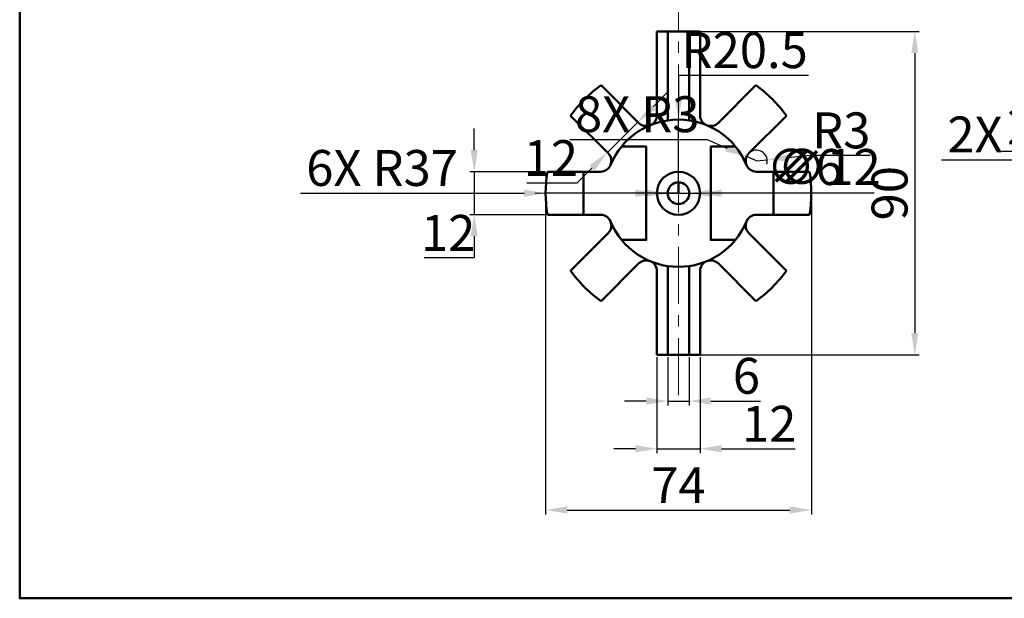
# Model space of a CAD drawing. Units: millimetres. Extents: x 147 to 984, y -369 to 435.
# Tile 1 of 10: x 147 to 422, y -369 to -208. Entities that reach past the tile are written whole.
import ezdxf

# ---------------------------------------------------------------- set-up
doc = ezdxf.new("R2010")
doc.units = ezdxf.units.MM
doc.header["$LTSCALE"] = 0.5
doc.linetypes.add('CENTER', pattern=[50.8, 31.75, -6.35, 6.35, -6.35])
for name, color, linetype, lineweight in [('M-CNTR', 1, 'CENTER', 18), ('M-DIMS', 2, 'Continuous', 25), ('M-OUTL', 7, 'Continuous', 50)]:
    doc.layers.add(name, color=color, linetype=linetype, lineweight=lineweight)
doc.styles.get("Standard").update_dxf_attribs({"font": 'arial.ttf'})
doc.dimstyles.new('ISO-25', dxfattribs={"dimtxt": 10, "dimasz": 6, "dimexe": 1.25, "dimexo": 0.625, "dimtad": 1, "dimtoh": 1, "dimdec": 0, "dimtxsty": 'Standard', "dimcen": 2.5, "dimadec": 0, "dimazin": 0, "dimtfac": 1, "dimtdec": 0, "dimtmove": 0, "dimatfit": 3, "dimfxl": 1, "dimarcsym": 0})

# ---------------------------------------------------------------- blocks, each defined once
blk = doc.blocks.new('*U94')
at = {"layer": 'M-CNTR', "color": 0, "transparency": 16777216}
blk.add_line((0, -186.27), (0, 51.67), dxfattribs=at)
blk = doc.blocks.new('*D112')
at = {"layer": 'Defpoints', "color": 0, "ltscale": 0.5, "transparency": 16777216}
for p in [(330.85, -211.73), (330.85, -301.73), (396.67, -301.73)]:
    blk.add_point(p, dxfattribs=at)
at = {"layer": 'M-DIMS', "color": 0, "lineweight": -2, "ltscale": 0.5, "transparency": 16777216}
for p, q in [((331.47, -211.73), (397.92, -211.73)), ((396.67, -217.73), (396.67, -295.73)), ((331.47, -301.73), (397.92, -301.73))]:
    blk.add_line(p, q, dxfattribs=at)
at = {"layer": 'M-DIMS', "color": 0, "ltscale": 0.5, "transparency": 16777216}
for points in [[(395.67, -217.73), (397.67, -217.73), (396.67, -211.73)], [(395.67, -295.73), (397.67, -295.73), (396.67, -301.73)]]:
    blk.add_solid(points, dxfattribs=at)
at = {"layer": 'M-DIMS', "color": 0, "ltscale": 0.5, "transparency": 16777216, "insert": (390.94, -256.73), "char_height": 10, "attachment_point": 5, "rotation": 90}
blk.add_mtext('90', dxfattribs=at)
blk = doc.blocks.new('*D113')
at = {"layer": 'Defpoints', "color": 0, "ltscale": 0.5, "transparency": 16777216}
for p in [(294.34, -250.73), (273.95, -262.73), (294.34, -262.73)]:
    blk.add_point(p, dxfattribs=at)
at = {"layer": 'M-DIMS', "color": 0, "lineweight": -2, "ltscale": 0.5, "transparency": 16777216}
for p, q in [((273.95, -244.73), (273.95, -238.73)), ((293.71, -250.73), (272.7, -250.73)), ((273.95, -250.73), (273.95, -262.73)), ((293.71, -262.73), (272.7, -262.73)), ((273.95, -268.73), (273.95, -274.73)), ((273.95, -274.73), (260.04, -274.73))]:
    blk.add_line(p, q, dxfattribs=at)
at = {"layer": 'M-DIMS', "color": 0, "ltscale": 0.5, "transparency": 16777216}
for points in [[(272.95, -244.73), (274.95, -244.73), (273.95, -250.73)], [(272.95, -268.73), (274.95, -268.73), (273.95, -262.73)]]:
    blk.add_solid(points, dxfattribs=at)
at = {"layer": 'M-DIMS', "color": 0, "ltscale": 0.5, "transparency": 16777216, "insert": (266.69, -269.08), "char_height": 10, "attachment_point": 5}
blk.add_mtext('12', dxfattribs=at)
blk = doc.blocks.new('*D114')
at = {"layer": 'Defpoints', "color": 0, "ltscale": 0.5, "transparency": 16777216}
for p in [(327.85, -301.73), (333.85, -301.73), (333.85, -314.59)]:
    blk.add_point(p, dxfattribs=at)
at = {"layer": 'M-DIMS', "color": 0, "lineweight": -2, "ltscale": 0.5, "transparency": 16777216}
for p, q in [((327.85, -302.35), (327.85, -315.84)), ((333.85, -302.35), (333.85, -315.84)), ((321.85, -314.59), (315.85, -314.59)), ((327.85, -314.59), (333.85, -314.59)), ((339.85, -314.59), (353.7, -314.59))]:
    blk.add_line(p, q, dxfattribs=at)
at = {"layer": 'M-DIMS', "color": 0, "ltscale": 0.5, "transparency": 16777216}
for points in [[(321.85, -313.59), (321.85, -315.59), (327.85, -314.59)], [(339.85, -313.59), (339.85, -315.59), (333.85, -314.59)]]:
    blk.add_solid(points, dxfattribs=at)
at = {"layer": 'M-DIMS', "color": 0, "ltscale": 0.5, "transparency": 16777216, "insert": (349.77, -308.86), "char_height": 10, "attachment_point": 5}
blk.add_mtext('6', dxfattribs=at)
blk = doc.blocks.new('*D115')
at = {"layer": 'Defpoints', "color": 0, "ltscale": 0.5, "transparency": 16777216}
for p in [(324.85, -301.73), (336.85, -301.73), (336.85, -327.86)]:
    blk.add_point(p, dxfattribs=at)
at = {"layer": 'M-DIMS', "color": 0, "lineweight": -2, "ltscale": 0.5, "transparency": 16777216}
for p, q in [((324.85, -302.35), (324.85, -329.11)), ((336.85, -302.35), (336.85, -329.11)), ((318.85, -327.86), (312.85, -327.86)), ((324.85, -327.86), (336.85, -327.86)), ((342.85, -327.86), (363.38, -327.86))]:
    blk.add_line(p, q, dxfattribs=at)
at = {"layer": 'M-DIMS', "color": 0, "ltscale": 0.5, "transparency": 16777216}
for points in [[(318.85, -326.86), (318.85, -328.86), (324.85, -327.86)], [(342.85, -326.86), (342.85, -328.86), (336.85, -327.86)]]:
    blk.add_solid(points, dxfattribs=at)
at = {"layer": 'M-DIMS', "color": 0, "ltscale": 0.5, "transparency": 16777216, "insert": (356.11, -322.22), "char_height": 10, "attachment_point": 5}
blk.add_mtext('12', dxfattribs=at)
blk = doc.blocks.new('*D116')
at = {"layer": 'Defpoints', "color": 0, "ltscale": 0.5, "transparency": 16777216}
for p in [(293.85, -256.73), (367.85, -256.73), (367.85, -344.92)]:
    blk.add_point(p, dxfattribs=at)
at = {"layer": 'M-DIMS', "color": 0, "lineweight": -2, "ltscale": 0.5, "transparency": 16777216}
for p, q in [((293.85, -257.35), (293.85, -346.17)), ((367.85, -257.35), (367.85, -346.17)), ((299.85, -344.92), (361.85, -344.92))]:
    blk.add_line(p, q, dxfattribs=at)
at = {"layer": 'M-DIMS', "color": 0, "ltscale": 0.5, "transparency": 16777216}
for points in [[(299.85, -343.92), (299.85, -345.92), (293.85, -344.92)], [(361.85, -343.92), (361.85, -345.92), (367.85, -344.92)]]:
    blk.add_solid(points, dxfattribs=at)
at = {"layer": 'M-DIMS', "color": 0, "ltscale": 0.5, "transparency": 16777216, "insert": (330.85, -339.3), "char_height": 10, "attachment_point": 5}
blk.add_mtext('74', dxfattribs=at)
blk = doc.blocks.new('*D117')
at = {"layer": 'Defpoints', "color": 0, "ltscale": 0.5, "transparency": 16777216}
for p in [(352.56, -247.74), (355.55, -247.45)]:
    blk.add_point(p, dxfattribs=at)
at = {"layer": 'M-DIMS', "color": 0, "lineweight": -2, "ltscale": 0.5, "transparency": 16777216}
for p, q in [((367.49, -246.27), (361.52, -246.86)), ((384.24, -246.27), (367.49, -246.27)), ((352.56, -247.74), (355.55, -247.45))]:
    blk.add_line(p, q, dxfattribs=at)
blk.add_arc((352.56, -247.74), 3, 341.7807, 123.0634, dxfattribs=at)
at = {"layer": 'M-DIMS', "color": 0, "ltscale": 0.5, "transparency": 16777216}
blk.add_solid([(361.42, -245.86), (361.62, -247.85), (355.55, -247.45)], dxfattribs=at)
at = {"layer": 'M-DIMS', "color": 0, "ltscale": 0.5, "transparency": 16777216, "insert": (376.18, -240.53), "char_height": 10, "attachment_point": 5}
blk.add_mtext('R3', dxfattribs=at)
blk = doc.blocks.new('*U118')
at = {"layer": 'M-CNTR', "color": 0, "transparency": 16777216}
blk.add_line((75.96, 0), (-10.9, 0), dxfattribs=at)
blk = doc.blocks.new('*D149')
at = {"layer": 'Defpoints', "color": 0, "ltscale": 0.5, "transparency": 16777216}
for p in [(309.27, -226.67), (300.79, -235.16), (311.04, -245.41)]:
    blk.add_point(p, dxfattribs=at)
at = {"layer": 'M-DIMS', "color": 0, "lineweight": -2, "ltscale": 0.5, "transparency": 16777216}
for p, q in [((309.71, -227.11), (320.41, -237.81)), ((323.77, -232.68), (328.01, -228.44)), ((301.23, -235.6), (311.92, -246.29)), ((319.53, -236.92), (311.04, -245.41)), ((306.8, -249.65), (302.56, -253.89)), ((302.56, -253.89), (288.65, -253.89))]:
    blk.add_line(p, q, dxfattribs=at)
at = {"layer": 'M-DIMS', "color": 0, "ltscale": 0.5, "transparency": 16777216}
for points in [[(323.06, -231.97), (324.48, -233.39), (319.53, -236.92)], [(306.09, -248.94), (307.5, -250.36), (311.04, -245.41)]]:
    blk.add_solid(points, dxfattribs=at)
at = {"layer": 'M-DIMS', "color": 0, "ltscale": 0.5, "transparency": 16777216, "insert": (295.29, -248.25), "char_height": 10, "attachment_point": 5}
blk.add_mtext('12', dxfattribs=at)
blk = doc.blocks.new('*D182')
at = {"layer": 'Defpoints', "color": 0, "ltscale": 0.5, "transparency": 16777216}
for p in [(293.85, -256.73), (330.85, -256.73)]:
    blk.add_point(p, dxfattribs=at)
at = {"layer": 'M-DIMS', "color": 0, "lineweight": -2, "ltscale": 0.5, "transparency": 16777216}
for p, q in [((225.57, -256.73), (271.63, -256.73)), ((271.63, -256.73), (287.85, -256.73)), ((330.85, -256.73), (293.85, -256.73))]:
    blk.add_line(p, q, dxfattribs=at)
at = {"layer": 'M-DIMS', "color": 0, "ltscale": 0.5, "transparency": 16777216}
blk.add_solid([(287.85, -255.73), (287.85, -257.73), (293.85, -256.73)], dxfattribs=at)
at = {"layer": 'M-DIMS', "color": 0, "ltscale": 0.5, "transparency": 16777216, "insert": (248.29, -251), "char_height": 10, "attachment_point": 5}
blk.add_mtext('6X R37', dxfattribs=at)
blk = doc.blocks.new('*D183')
at = {"layer": 'Defpoints', "color": 0, "ltscale": 0.5, "transparency": 16777216}
for p in [(330.85, -236.23), (330.85, -256.73)]:
    blk.add_point(p, dxfattribs=at)
at = {"layer": 'M-DIMS', "color": 0, "lineweight": -2, "ltscale": 0.5, "transparency": 16777216}
for p, q in [((367.09, -223.93), (330.85, -223.93)), ((330.85, -223.93), (330.85, -230.23)), ((330.85, -256.73), (330.85, -236.23))]:
    blk.add_line(p, q, dxfattribs=at)
at = {"layer": 'M-DIMS', "color": 0, "ltscale": 0.5, "transparency": 16777216}
blk.add_solid([(329.85, -230.23), (331.85, -230.23), (330.85, -236.23)], dxfattribs=at)
at = {"layer": 'M-DIMS', "color": 0, "ltscale": 0.5, "transparency": 16777216, "insert": (349.28, -218.2), "char_height": 10, "attachment_point": 5}
blk.add_mtext('R20.5', dxfattribs=at)
blk = doc.blocks.new('*D184')
at = {"layer": 'Defpoints', "color": 0, "ltscale": 0.5, "transparency": 16777216}
for p in [(349.81, -246.55), (352.56, -247.74)]:
    blk.add_point(p, dxfattribs=at)
at = {"layer": 'M-DIMS', "color": 0, "lineweight": -2, "ltscale": 0.5, "transparency": 16777216}
for p, q in [((300.55, -241.77), (338.8, -241.77)), ((338.8, -241.77), (344.31, -244.16)), ((352.56, -247.74), (349.81, -246.55))]:
    blk.add_line(p, q, dxfattribs=at)
at = {"layer": 'M-DIMS', "color": 0, "ltscale": 0.5, "transparency": 16777216}
blk.add_solid([(344.7, -243.24), (343.91, -245.08), (349.81, -246.55)], dxfattribs=at)
at = {"layer": 'M-DIMS', "color": 0, "ltscale": 0.5, "transparency": 16777216, "insert": (319.36, -236.03), "char_height": 10, "attachment_point": 5}
blk.add_mtext('8X R3', dxfattribs=at)
blk = doc.blocks.new('*D185')
at = {"layer": 'Defpoints', "color": 0, "ltscale": 0.5, "transparency": 16777216}
for p in [(324.85, -256.73), (336.85, -256.73)]:
    blk.add_point(p, dxfattribs=at)
at = {"layer": 'M-DIMS', "color": 0, "lineweight": -2, "ltscale": 0.5, "transparency": 16777216}
for p, q in [((318.85, -256.73), (312.85, -256.73)), ((324.85, -256.73), (336.85, -256.73)), ((359.62, -256.73), (342.85, -256.73)), ((385.34, -256.73), (359.62, -256.73))]:
    blk.add_line(p, q, dxfattribs=at)
at = {"layer": 'M-DIMS', "color": 0, "ltscale": 0.5, "transparency": 16777216}
for points in [[(318.85, -255.73), (318.85, -257.73), (324.85, -256.73)], [(342.85, -255.73), (342.85, -257.73), (336.85, -256.73)]]:
    blk.add_solid(points, dxfattribs=at)
at = {"layer": 'M-DIMS', "color": 0, "ltscale": 0.5, "transparency": 16777216, "insert": (372.79, -250.72), "char_height": 10, "attachment_point": 5}
blk.add_mtext('∅12', dxfattribs=at)
blk = doc.blocks.new('*D186')
at = {"layer": 'Defpoints', "color": 0, "ltscale": 0.5, "transparency": 16777216}
for p in [(327.85, -256.73), (333.85, -256.73)]:
    blk.add_point(p, dxfattribs=at)
at = {"layer": 'M-DIMS', "color": 0, "lineweight": -2, "ltscale": 0.5, "transparency": 16777216}
for p, q in [((321.85, -256.73), (315.85, -256.73)), ((327.85, -256.73), (333.85, -256.73)), ((356.62, -256.73), (339.85, -256.73)), ((374.67, -256.73), (356.62, -256.73))]:
    blk.add_line(p, q, dxfattribs=at)
at = {"layer": 'M-DIMS', "color": 0, "ltscale": 0.5, "transparency": 16777216}
for points in [[(321.85, -255.73), (321.85, -257.73), (327.85, -256.73)], [(339.85, -255.73), (339.85, -257.73), (333.85, -256.73)]]:
    blk.add_solid(points, dxfattribs=at)
at = {"layer": 'M-DIMS', "color": 0, "ltscale": 0.5, "transparency": 16777216, "insert": (365.96, -250.72), "char_height": 10, "attachment_point": 5}
blk.add_mtext('∅6', dxfattribs=at)
blk = doc.blocks.new('*D187')
at = {"layer": 'Defpoints', "color": 0, "ltscale": 0.5, "transparency": 16777216}
for p in [(458.81, -255.82), (465.95, -262.83)]:
    blk.add_point(p, dxfattribs=at)
at = {"layer": 'M-DIMS', "color": 0, "lineweight": -2, "ltscale": 0.5, "transparency": 16777216}
for p, q in [((404.11, -247.4), (450.26, -247.4)), ((450.26, -247.4), (454.54, -251.61)), ((465.95, -262.83), (458.81, -255.82))]:
    blk.add_line(p, q, dxfattribs=at)
at = {"layer": 'M-DIMS', "color": 0, "ltscale": 0.5, "transparency": 16777216}
blk.add_solid([(455.24, -250.9), (453.83, -252.32), (458.81, -255.82)], dxfattribs=at)
at = {"layer": 'M-DIMS', "color": 0, "ltscale": 0.5, "transparency": 16777216, "insert": (426.87, -241.67), "char_height": 10, "attachment_point": 5}
blk.add_mtext('2X R10', dxfattribs=at)
blk = doc.blocks.new('*D188')
at = {"layer": 'Defpoints', "color": 0, "ltscale": 0.5, "transparency": 16777216}
for p in [(463.47, -256.28), (465.95, -262.83)]:
    blk.add_point(p, dxfattribs=at)
at = {"layer": 'M-DIMS', "color": 0, "lineweight": -2, "ltscale": 0.5, "transparency": 16777216}
for p, q in [((420.81, -245.06), (459.22, -245.06)), ((459.22, -245.06), (461.34, -250.67)), ((465.95, -262.83), (463.47, -256.28))]:
    blk.add_line(p, q, dxfattribs=at)
at = {"layer": 'M-DIMS', "color": 0, "ltscale": 0.5, "transparency": 16777216}
blk.add_solid([(462.28, -250.31), (460.41, -251.02), (463.47, -256.28)], dxfattribs=at)
at = {"layer": 'M-DIMS', "color": 0, "ltscale": 0.5, "transparency": 16777216, "insert": (439.7, -239.41), "char_height": 10, "attachment_point": 5}
blk.add_mtext('2X R7', dxfattribs=at)

msp = doc.modelspace()

# ---------------------------------------------------------------- linework, layer by layer
at = {"layer": 'M-OUTL', "ltscale": 0.5}
for p, q in [((336.8467, -211.7297), (324.8467, -211.7297)), ((324.8467, -211.7297), (324.8467, -235.0214)), ((327.8467, -211.7297), (327.8467, -236.4504)), ((330.8467, -211.7297), (336.8467, -211.7297)), ((333.8467, -211.7297), (333.8467, -236.4504)), ((336.8467, -211.7297), (336.8467, -235.0214)), ((324.8467, -235.0214), (324.8467, -220.2194)), ((336.8467, -235.0214), (336.8467, -220.2194)), ((319.7393, -237.1369), (309.2727, -226.6704)), ((341.9541, -237.1369), (352.4207, -226.6704)), ((311.254, -245.6222), (300.7874, -235.1556)), ((350.4394, -245.6222), (360.906, -235.1556)), ((309.1384, -250.7297), (294.3364, -250.7297)), ((304.3467, -250.7297), (304.3467, -262.7297)), ((367.357, -250.7297), (352.555, -250.7297)), ((352.555, -250.7297), (367.357, -250.7297)), ((357.3467, -250.7297), (357.3467, -262.7297)), ((330.8467, -256.7297), (330.8467, -253.7297)), ((309.1384, -262.7297), (294.3364, -262.7297)), ((367.357, -262.7297), (352.555, -262.7297)), ((352.555, -262.7297), (367.357, -262.7297)), ((311.254, -267.8371), (300.7874, -278.3037)), ((350.4394, -267.8371), (360.906, -278.3037)), ((319.7393, -276.3224), (309.2727, -286.789)), ((341.9541, -276.3224), (352.4207, -286.789)), ((324.8467, -301.7297), (324.8467, -278.438)), ((327.8467, -301.7297), (327.8467, -277.009)), ((333.8467, -301.7297), (333.8467, -277.009)), ((336.8467, -301.7297), (336.8467, -278.438)), ((336.8467, -301.7297), (324.8467, -301.7297)), ((336.8467, -301.7297), (324.8467, -301.7297))]:
    msp.add_line(p, q, dxfattribs=at)
msp.add_lwpolyline([(147.3511, 435.3078), (984.0884, 435.3078), (984.0884, -369.4968), (147.3511, -369.4968)], close=True, dxfattribs=at)
for points in [[(314.9958, -243.7297), (321.8467, -243.7297), (321.8467, -256.7297), (321.8467, -269.7297), (314.9958, -269.7297)], [(346.6976, -243.7297), (339.8467, -243.7297), (339.8467, -256.7297), (339.8467, -269.7297), (346.6976, -269.7297)]]:
    msp.add_lwpolyline(points, dxfattribs=at)
for radius in [6, 3]:
    msp.add_circle((330.8467, -256.7297), radius, dxfattribs=at)
for centre, radius, start, end in [((330.8467, -256.7297), 37, 125.667582, 144.332418), ((330.8467, -256.7297), 37, 35.667582, 54.332418), ((321.8467, -235.0214), 3, 292.518314, 0), ((321.8467, -235.0214), 3, 292.518314, 0), ((339.8467, -235.0214), 3, 180, 247.481686), ((339.8467, -235.0214), 3, 180, 247.481686), ((330.8467, -256.7297), 20.5, 22.481686, 157.518314), ((321.8606, -235.0156), 3, 225, 292.481686), ((339.8328, -235.0156), 3, 247.518314, 315), ((309.1327, -247.7435), 3, 337.518314, 45), ((352.5608, -247.7435), 3, 135, 202.481686), ((309.1384, -247.7297), 3, 270, 337.481686), ((352.555, -247.7297), 3, 202.518314, 270), ((352.555, -247.7297), 3, 202.518314, 270), ((330.8467, -256.7297), 37, 170.667582, 189.332418), ((330.8467, -256.7297), 37, 350.667582, 9.332418), ((330.8467, -256.7297), 37, 350.667582, 9.332418), ((309.1384, -265.7297), 3, 22.518314, 90), ((352.555, -265.7297), 3, 90, 157.481686), ((352.555, -265.7297), 3, 90, 157.481686), ((309.1327, -265.7158), 3, 315, 22.481686), ((330.8467, -256.7297), 20.5, 202.481686, 337.518314), ((352.5608, -265.7158), 3, 157.518314, 225), ((321.8606, -278.4437), 3, 67.518314, 135), ((321.8467, -278.438), 3, 0, 67.481686), ((339.8467, -278.438), 3, 112.518314, 180), ((339.8328, -278.4437), 3, 45, 112.481686), ((330.8467, -256.7297), 37, 215.667582, 234.332418), ((330.8467, -256.7297), 37, 305.667582, 324.332418)]:
    msp.add_arc(centre, radius, start, end, dxfattribs=at)

# ---------------------------------------------------------------- block references
at = {"layer": 'M-CNTR'}
for name, p in [('*U94', (330.8467, -126.6547)), ('*U118', (301.7374, -256.7297))]:
    msp.add_blockref(name, p, dxfattribs=at)

# ---------------------------------------------------------------- dimensions: what is measured, and where the dimension line sits
at = {"layer": 'M-DIMS', "ltscale": 0.5}
dim = msp.add_radius_dim(center=(330.8467, -256.7297), mpoint=(330.847, -236.2297), dimstyle='ISO-25', override={"dimdec": 1, "dimlfac": 1, "dimrnd": 0, "dimzin": 0, "dimdsep": 46, "dimlunit": 2}, dxfattribs=at)
dim.commit()
dim.dimension.update_dxf_attribs({"geometry": '*D183', "text_midpoint": (349.2825, -223.9297), "dimtype": 164})
for base, p1, p2, angle, override, picture, middle in [((396.6712, -301.7297), (330.8467, -211.7297), (330.8467, -301.7297), 90, {"dimclrd": 0, "dimclre": 0, "dimclrt": 0}, '*D112', (390.9405, -256.7297)), ((311.0405, -245.4087), (309.2727, -226.6704), (300.7874, -235.1556), 225, {"dimdec": 0, "dimlfac": 1, "dimrnd": 0, "dimzin": 0, "dimdsep": 46, "dimlunit": 2}, '*D149', (295.2897, -248.2485)), ((273.9506, -262.7297), (294.3364, -250.7297), (294.3364, -262.7297), 90, {"dimclrd": 0, "dimclre": 0, "dimclrt": 0}, '*D113', (266.6851, -269.0842))]:
    dim = msp.add_linear_dim(base=base, p1=p1, p2=p2, angle=angle, dimstyle='ISO-25', override=override, dxfattribs=at)
    dim.commit()
    dim.dimension.update_dxf_attribs({"geometry": picture, "text_midpoint": middle})
for center, mpoint, text, picture, middle in [((352.5608, -247.7435), (349.8091, -246.5484), '8X <>', '*D184', (319.3643, -236.0338)), ((465.9465, -262.8255), (463.4671, -256.2793), '2X <>', '*D188', (439.7002, -239.4084)), ((465.9465, -262.8255), (458.8145, -255.8159), '2X <>', '*D187', (426.8718, -241.6737)), ((330.8467, -256.7297), (293.8467, -256.73), '6X <>', '*D182', (248.2851, -250.9961))]:
    dim = msp.add_radius_dim(center=center, mpoint=mpoint, text=text, dimstyle='ISO-25', override={"dimdec": 0, "dimlfac": 1, "dimrnd": 0, "dimzin": 0, "dimdsep": 46, "dimlunit": 2}, dxfattribs=at)
    dim.commit()
    dim.dimension.update_dxf_attribs({"geometry": picture, "text_midpoint": middle})
dim = msp.add_radius_dim(center=(352.5608, -247.7435), mpoint=(355.5462, -247.448), dimstyle='ISO-25', override={"dimclrd": 0, "dimclre": 0, "dimclrt": 0}, dxfattribs=at)
dim.commit()
dim.dimension.update_dxf_attribs({"geometry": '*D117', "text_midpoint": (376.1755, -240.5316)})
for p1, p2, picture, middle in [((324.8467, -256.7293), (336.8467, -256.73), '*D185', (359.6175, -256.7313)), ((327.8467, -256.7293), (333.8467, -256.73), '*D186', (356.6175, -256.7325))]:
    dim = msp.add_diameter_dim_2p(p1=p1, p2=p2, dimstyle='ISO-25', override={"dimdec": 0, "dimlfac": 1, "dimrnd": 0, "dimzin": 0, "dimdsep": 46, "dimlunit": 2}, dxfattribs=at)
    dim.commit()
    dim.dimension.update_dxf_attribs({"geometry": picture, "text_midpoint": middle, "dimtype": 163})
for base, p1, p2, picture, middle in [((367.8467, -344.9244), (293.8467, -256.7297), (367.8467, -256.7297), '*D116', (330.8467, -339.2994)), ((336.8467, -327.8638), (324.8467, -301.7297), (336.8467, -301.7297), '*D115', (356.1122, -322.2184)), ((333.8467, -314.5941), (327.8467, -301.7297), (333.8467, -301.7297), '*D114', (349.7732, -308.8633))]:
    dim = msp.add_linear_dim(base=base, p1=p1, p2=p2, dimstyle='ISO-25', override={"dimclrd": 0, "dimclre": 0, "dimclrt": 0}, dxfattribs=at)
    dim.commit()
    dim.dimension.update_dxf_attribs({"geometry": picture, "text_midpoint": middle})

doc.saveas('drawing.dxf')
